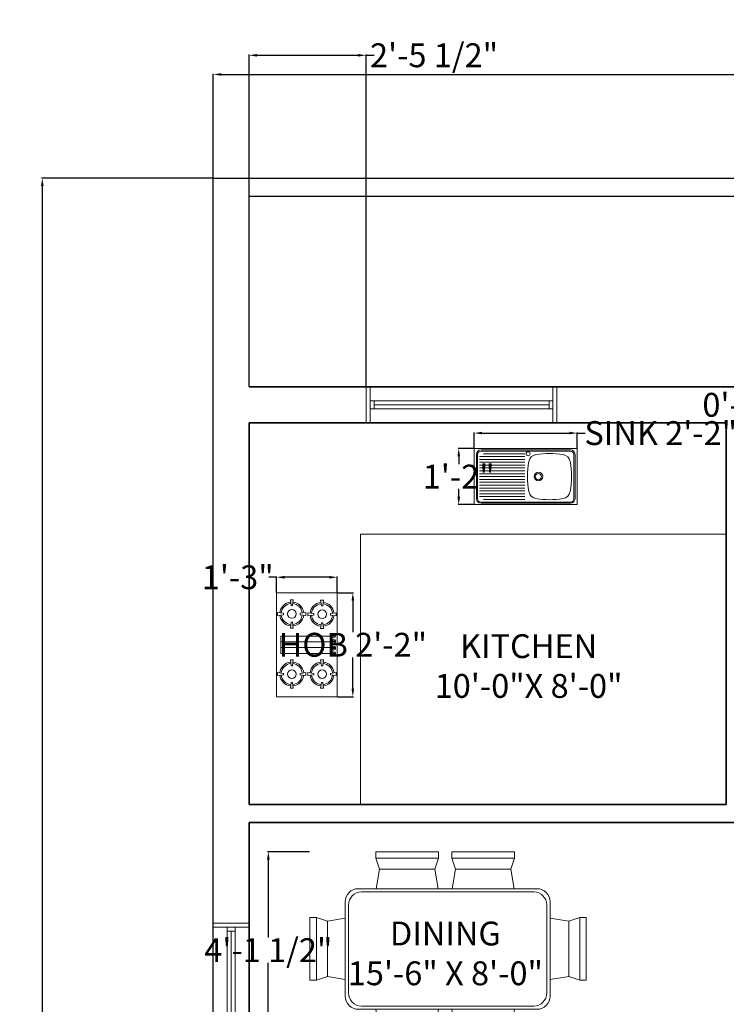
# Model space of a CAD drawing. Units: inches. Extents: x 84 to 590, y 32 to 648.
# Tile 5 of 6: x 84 to 262, y 401 to 648. Entities that reach past the tile are written whole.
import ezdxf

# ---------------------------------------------------------------- set-up
doc = ezdxf.new("R2010")
doc.units = ezdxf.units.IN
doc.header["$MEASUREMENT"] = 0
for name, color, linetype, lineweight in [('A-ANNO-DIMS', 2, 'Continuous', 18), ('A-AREA-IDEN', 7, 'Continuous', 18), ('A-EQPM', 9, 'Continuous', 18), ('A-FLOR-CASE', 9, 'Continuous', 18), ('A-FLOR-FIXT', 9, 'Continuous', 18), ('A-FURN', 8, 'Continuous', 18), ('A-GLAZ', 4, 'Continuous', 18), ('A-WALL', 7, 'Continuous', 35), ('C-PROP', 7, 'Continuous', 30)]:
    doc.layers.add(name, color=color, linetype=linetype, lineweight=lineweight)
doc.styles.get("Standard").update_dxf_attribs({"font": 'arial.ttf'})
doc.dimstyles.get("Standard").update_dxf_attribs({"dimtxt": 6, "dimasz": 2, "dimexe": 0.18, "dimexo": 0.0625, "dimgap": 0.09, "dimtad": 0, "dimtih": 1, "dimtoh": 1, "dimdec": 0, "dimzin": 0, "dimdsep": 46, "dimlunit": 4, "dimtxsty": 'Standard', "dimcen": 0.09, "dimadec": 0, "dimazin": 0, "dimtfac": 1, "dimtdec": 0, "dimtofl": 0, "dimtmove": 0, "dimatfit": 3, "dimfxl": 1, "dimtolj": 1, "dimtzin": 0, "dimarcsym": 1})

# ---------------------------------------------------------------- blocks, each defined once
blk = doc.blocks.new('A$C6C037A94')
for p, q in [((0.7877, 1.6959), (0.4032, 1.6959)), ((0.4032, 1.6959), (0.4039, 1.6557)), ((0.7877, 1.6557), (0.7877, 1.6959)), ((0.4258, 1.588), (0.4039, 1.6557)), ((0.7877, 1.6557), (0.4039, 1.6557)), ((0.7658, 1.588), (0.7877, 1.6557)), ((0.407, 1.4737), (0.4258, 1.588)), ((0.7658, 1.588), (0.4258, 1.588)), ((0.7847, 1.4737), (0.7658, 1.588)), ((0.307, 1.4737), (0.8868, 1.4737)), ((0.327, 1.4537), (0.8668, 1.4537)), ((0.227, 0.2974), (0.227, 1.3937)), ((0.9668, 1.3937), (0.9668, 0.2974)), ((0.247, 0.3174), (0.247, 1.3737)), ((0.9468, 1.3737), (0.9468, 0.3174)), ((0, 1.2552), (0, 0.8707)), ((0.0402, 1.2552), (0, 1.2552)), ((0.0402, 1.2552), (0.0402, 0.8714)), ((0.1079, 1.2333), (0.0402, 1.2552)), ((0.227, 1.2529), (0.1079, 1.2333)), ((0.1079, 1.2333), (0.1079, 0.8933)), ((0.9668, 1.2553), (1.1005, 1.2333)), ((1.1005, 1.2333), (1.1682, 1.2552)), ((1.1005, 1.2333), (1.1005, 0.8933)), ((1.1682, 1.2552), (1.2084, 1.2552)), ((1.1682, 1.2552), (1.1682, 0.8714)), ((1.2084, 1.2552), (1.2084, 0.8707)), ((0, 0.8707), (0.0402, 0.8714)), ((0.1079, 0.8933), (0.0402, 0.8714)), ((0.227, 0.8736), (0.1079, 0.8933)), ((0.9668, 0.8712), (1.1005, 0.8933)), ((1.1005, 0.8933), (1.1682, 0.8714)), ((1.2084, 0.8707), (1.1682, 0.8714)), ((0, 0.7888), (0, 0.4043)), ((0.0402, 0.7888), (0, 0.7888)), ((0.0402, 0.7888), (0.0402, 0.405)), ((0.1079, 0.7669), (0.0402, 0.7888)), ((0.227, 0.7865), (0.1079, 0.7669)), ((0.9668, 0.7889), (1.1005, 0.7669)), ((1.1005, 0.7669), (1.1682, 0.7888)), ((1.1682, 0.7888), (1.1682, 0.405)), ((1.1682, 0.7888), (1.2084, 0.7888)), ((1.2084, 0.7888), (1.2084, 0.4043)), ((0.1079, 0.7669), (0.1079, 0.4269)), ((1.1005, 0.7669), (1.1005, 0.4269)), ((0.1079, 0.4269), (0.0402, 0.405)), ((0.227, 0.4072), (0.1079, 0.4269)), ((0.9668, 0.4048), (1.1005, 0.4269)), ((1.1005, 0.4269), (1.1682, 0.405)), ((0, 0.4043), (0.0402, 0.405)), ((1.2084, 0.4043), (1.1682, 0.405)), ((0.8868, 0.2174), (0.307, 0.2174)), ((0.8668, 0.2374), (0.327, 0.2374)), ((0.4078, 0.2174), (0.4258, 0.1079)), ((0.7839, 0.2174), (0.7658, 0.1079)), ((0.4258, 0.1079), (0.4039, 0.0402)), ((0.7658, 0.1079), (0.4258, 0.1079)), ((0.7658, 0.1079), (0.7877, 0.0402)), ((0.4032, 0), (0.4039, 0.0402)), ((0.7877, 0), (0.4032, 0)), ((0.7877, 0.0402), (0.4039, 0.0402)), ((0.7877, 0.0402), (0.7877, 0))]:
    blk.add_line(p, q)
for centre, start, end in [((0.307, 1.3937), 90, 180), ((0.327, 1.3737), 90, 180), ((0.8668, 1.3737), 360, 90), ((0.8868, 1.3937), 360, 90), ((0.327, 0.3174), 180, 270), ((0.8668, 0.3174), 270, 0), ((0.307, 0.2974), 180, 270), ((0.8868, 0.2974), 270, 360)]:
    blk.add_arc(centre, 0.08, start, end)
blk = doc.blocks.new('A$C57CF26DA')
for p, q in [((0, 0), (0, 420)), ((720, 420), (0, 420)), ((166.9, 413), (146.9, 413)), ((146.9, 413), (151.9, 373)), ((161.9, 373), (166.9, 413)), ((583.6, 413), (563.6, 413)), ((563.6, 413), (568.6, 373)), ((578.6, 373), (583.6, 413)), ((720, 0), (720, 420)), ((151.9, 373), (161.9, 373)), ((300, 390.9), (300, 49.1)), ((300, 390.9), (420, 390.9)), ((340, 390.9), (340, 49.1)), ((380, 390.9), (380, 49.1)), ((420, 390.9), (420, 49.1)), ((568.6, 373), (578.6, 373)), ((98.9, 320), (58.9, 325)), ((58.9, 325), (58.9, 305)), ((58.9, 305), (98.9, 310)), ((98.9, 310), (98.9, 320)), ((254.8, 325), (214.8, 320)), ((214.8, 320), (214.8, 310)), ((214.8, 310), (254.8, 305)), ((254.8, 305), (254.8, 325)), ((515.6, 320), (475.6, 325)), ((475.6, 325), (475.6, 305)), ((475.6, 305), (515.6, 310)), ((515.6, 310), (515.6, 320)), ((671.6, 325), (631.6, 320)), ((631.6, 320), (631.6, 310)), ((631.6, 310), (671.6, 305)), ((671.6, 305), (671.6, 325)), ((151.9, 257), (146.9, 217)), ((146.9, 217), (166.9, 217)), ((161.9, 257), (151.9, 257)), ((166.9, 217), (161.9, 257)), ((568.6, 257), (563.6, 217)), ((563.6, 217), (583.6, 217)), ((578.6, 257), (568.6, 257)), ((583.6, 217), (578.6, 257)), ((166.9, 203), (146.9, 203)), ((146.9, 203), (151.9, 163)), ((151.9, 163), (161.9, 163)), ((161.9, 163), (166.9, 203)), ((581.1, 203), (561.1, 203)), ((561.1, 203), (566.1, 163)), ((566.1, 163), (576.1, 163)), ((576.1, 163), (581.1, 203)), ((98.9, 110), (58.9, 115)), ((58.9, 115), (58.9, 95)), ((58.9, 95), (98.9, 100)), ((98.9, 100), (98.9, 110)), ((254.8, 115), (214.8, 110)), ((214.8, 110), (214.8, 100)), ((214.8, 100), (254.8, 95)), ((254.8, 95), (254.8, 115)), ((513.1, 110), (473.1, 115)), ((473.1, 115), (473.1, 95)), ((473.1, 95), (513.1, 100)), ((513.1, 100), (513.1, 110)), ((669, 115), (629, 110)), ((629, 110), (629, 100)), ((629, 100), (669, 95)), ((669, 95), (669, 115)), ((151.9, 47), (146.9, 7)), ((146.9, 7), (166.9, 7)), ((161.9, 47), (151.9, 47)), ((166.9, 7), (161.9, 47)), ((301.5, 38.7), (294.7, 38.7)), ((294.7, 38.7), (294.7, 11.3)), ((294.7, 11.3), (301.5, 11.3)), ((420, 49.1), (300, 49.1)), ((301.5, 11.3), (301.5, 38.7)), ((340.5, 38.7), (333.7, 38.7)), ((333.7, 38.7), (333.7, 11.3)), ((333.7, 11.3), (340.5, 11.3)), ((340.5, 11.3), (340.5, 38.7)), ((379.7, 11.3), (379.7, 38.7)), ((379.7, 38.7), (386.5, 38.7)), ((386.5, 11.3), (379.7, 11.3)), ((386.5, 38.7), (386.5, 11.3)), ((418.7, 11.3), (418.7, 38.7)), ((418.7, 38.7), (425.5, 38.7)), ((425.5, 11.3), (418.7, 11.3)), ((425.5, 38.7), (425.5, 11.3)), ((566.1, 47), (561.1, 7)), ((561.1, 7), (581.1, 7)), ((576.1, 47), (566.1, 47)), ((581.1, 7), (576.1, 47)), ((720, 0), (0, 0))]:
    blk.add_line(p, q)
for centre in [(156.9, 315), (573.6, 315), (156.9, 105), (571.1, 105)]:
    blk.add_circle(centre, 30)
for centre, radius, start, end in [((156.9, 315), 83, 95.58493, 174.41507), ((156.9, 315), 73, 95.37384, 174.62616), ((156.9, 315), 73, 5.37384, 84.62616), ((156.9, 315), 83, 5.58493, 84.41507), ((573.6, 315), 83, 95.58493, 174.41507), ((573.6, 315), 73, 95.37384, 174.62616), ((573.6, 315), 73, 5.37384, 84.62616), ((573.6, 315), 83, 5.58493, 84.41507), ((156.9, 315), 83, 185.58493, 264.41507), ((156.9, 315), 73, 185.37384, 264.62616), ((156.9, 315), 73, 275.37384, 354.62616), ((156.9, 315), 83, 275.58493, 354.41507), ((573.6, 315), 83, 185.58493, 264.41507), ((573.6, 315), 73, 185.37384, 264.62616), ((573.6, 315), 73, 275.37384, 354.62616), ((573.6, 315), 83, 275.58493, 354.41507), ((156.9, 105), 83, 95.58493, 174.41507), ((156.9, 105), 73, 95.37384, 174.62616), ((156.9, 105), 73, 5.37384, 84.62616), ((156.9, 105), 83, 5.58493, 84.41507), ((571.1, 105), 83, 95.58493, 174.41507), ((571.1, 105), 73, 95.37384, 174.62616), ((571.1, 105), 73, 5.37384, 84.62616), ((571.1, 105), 83, 5.58493, 84.41507), ((156.9, 105), 83, 185.58493, 264.41507), ((156.9, 105), 73, 185.37384, 264.62616), ((156.9, 105), 73, 275.37384, 354.62616), ((156.9, 105), 83, 275.58493, 354.41507), ((571.1, 105), 83, 185.58493, 264.41507), ((571.1, 105), 73, 185.37384, 264.62616), ((571.1, 105), 73, 275.37384, 354.62616), ((571.1, 105), 83, 275.58493, 354.41507), ((298.1, 25), 13.7, 104.47751, 255.52249), ((298.1, 25), 13.7, 284.47751, 75.52249), ((337.1, 25), 13.7, 104.47751, 255.52249), ((337.1, 25), 13.7, 284.47751, 75.52249), ((383.1, 25), 13.7, 104.47751, 255.52249), ((383.1, 25), 13.7, 284.47751, 75.52249), ((422.1, 25), 13.7, 104.47751, 255.52249), ((422.1, 25), 13.7, 284.47751, 75.52249)]:
    blk.add_arc(centre, radius, start, end)
blk = doc.blocks.new('A$C0C3933DC')
for p, q in [((0, 490), (0, 0)), ((900, 490), (0, 490)), ((19.5, 52.5), (19.5, 437.5)), ((29.5, 52.5), (29.5, 437.5)), ((59.5, 477.5), (450, 477.5)), ((59.5, 467.5), (450, 467.5)), ((441, 445), (80.7, 445)), ((840.5, 477.5), (450, 477.5)), ((840.5, 467.5), (450, 467.5)), ((870.5, 52.5), (870.5, 437.5)), ((880.5, 52.5), (880.5, 437.5)), ((900, 0), (900, 490)), ((441, 420), (45, 420)), ((441, 395), (45, 395)), ((441, 370), (45, 370)), ((441, 345), (45, 345)), ((441, 320), (45, 320)), ((441, 295), (45, 295)), ((441, 270), (45, 270)), ((441, 245), (45, 245)), ((441, 220), (45, 220)), ((441, 195), (45, 195)), ((441, 170), (45, 170)), ((441, 145), (45, 145)), ((441, 120), (45, 120)), ((441, 95), (45, 95)), ((0, 0), (900, 0)), ((441, 70), (45, 70)), ((450, 22.5), (59.5, 22.5)), ((450, 12.5), (59.5, 12.5)), ((441, 45), (80.7, 45)), ((450, 22.5), (840.5, 22.5)), ((450, 12.5), (840.5, 12.5))]:
    blk.add_line(p, q)
for centre, radius in [((471, 445), 17.5), ((561, 245), 38), ((561, 245), 27.5)]:
    blk.add_circle(centre, radius)
for centre, radius, start, end in [((59.5, 437.5), 40, 90, 180), ((59.5, 437.5), 30, 90, 180), ((551.5, 363.5), 75, 99.07872, 169.88522), ((658, -303), 750, 80.92128, 99.07872), ((764.5, 363.5), 75, 10.11478, 80.92128), ((840.5, 437.5), 40, 0, 90), ((840.5, 437.5), 30, 0, 90), ((1216, 245), 750, 169.88522, 190.11478), ((100, 245), 750, 349.88522, 10.11478), ((551.5, 126.5), 75, 190.11478, 260.92128), ((764.5, 126.5), 75, 279.07872, 349.88522), ((59.5, 52.5), 40, 180, 270), ((59.5, 52.5), 30, 180, 270), ((658, 793), 750, 260.92128, 279.07872), ((840.5, 52.5), 30, 270, 0), ((840.5, 52.5), 40, 270, 0)]:
    blk.add_arc(centre, radius, start, end)
blk = doc.blocks.new('*D12')
at = {"layer": 'A-ANNO-DIMS', "color": 0, "lineweight": -2, "transparency": 16777216}
for p, q in [((133.03, 608.4), (133.03, 634.6)), ((135.03, 634.42), (307.85, 634.42)), ((491.03, 634.42), (318.21, 634.42)), ((493.03, 608.4), (493.03, 634.6))]:
    blk.add_line(p, q, dxfattribs=at)
at = {"layer": 'A-ANNO-DIMS', "color": 0, "transparency": 16777216}
for points in [[(135.03, 634.75), (135.03, 634.08), (133.03, 634.42)], [(491.03, 634.75), (491.03, 634.08), (493.03, 634.42)]]:
    blk.add_solid(points, dxfattribs=at)
at = {"layer": 'Defpoints', "color": 0, "transparency": 16777216}
for p in [(493.03, 634.42), (133.03, 608.34), (493.03, 608.34)]:
    blk.add_point(p, dxfattribs=at)
at = {"layer": 'A-ANNO-DIMS', "color": 0, "transparency": 16777216, "insert": (313.03, 634.42), "char_height": 6, "attachment_point": 5}
blk.add_mtext("\\A1;30'", dxfattribs=at)
blk = doc.blocks.new('*D13')
at = {"layer": 'A-ANNO-DIMS', "color": 0, "lineweight": -2, "transparency": 16777216}
for p, q in [((132.97, 608.34), (89.87, 608.34)), ((90.05, 606.34), (90.05, 359.49)), ((90.05, 106.34), (90.05, 353.18)), ((132.97, 104.34), (89.87, 104.34))]:
    blk.add_line(p, q, dxfattribs=at)
at = {"layer": 'A-ANNO-DIMS', "color": 0, "transparency": 16777216}
for points in [[(89.71, 606.34), (90.38, 606.34), (90.05, 608.34)], [(89.71, 106.34), (90.38, 106.34), (90.05, 104.34)]]:
    blk.add_solid(points, dxfattribs=at)
at = {"layer": 'Defpoints', "color": 0, "transparency": 16777216}
for p in [(90.05, 608.34), (133.03, 608.34), (133.03, 104.34)]:
    blk.add_point(p, dxfattribs=at)
at = {"layer": 'A-ANNO-DIMS', "color": 0, "transparency": 16777216, "insert": (90.05, 356.34), "char_height": 6, "attachment_point": 5}
blk.add_mtext("\\A1;40'", dxfattribs=at)
blk = doc.blocks.new('WIND')
for p, q in [((-51.89, 1021.98), (-99.89, 1021.98)), ((-99.89, 1021.98), (-99.89, 1012.98)), ((-98.89, 1021.98), (-98.89, 1012.98)), ((-52.89, 1012.98), (-52.89, 1021.98)), ((-51.89, 1012.98), (-51.89, 1021.98)), ((-98.89, 1018.48), (-52.89, 1018.48)), ((-97.89, 1018.48), (-97.89, 1016.48)), ((-53.89, 1016.48), (-53.89, 1018.48)), ((-98.89, 1016.48), (-52.89, 1016.48)), ((-97.89, 1017.48), (-53.89, 1017.48)), ((-99.89, 1012.98), (-51.89, 1012.98))]:
    blk.add_line(p, q)
blk = doc.blocks.new('*D20')
at = {"layer": 'A-ANNO-DIMS', "color": 0, "lineweight": -2, "transparency": 16777216}
for p, q in [((274.33, 557.84), (274.33, 559.84)), ((277.86, 555.84), (274.15, 555.84)), ((277.86, 546.84), (274.15, 546.84)), ((274.33, 544.84), (274.33, 542.84))]:
    blk.add_line(p, q, dxfattribs=at)
at = {"layer": 'A-ANNO-DIMS', "color": 0, "transparency": 16777216}
for points in [[(273.99, 557.84), (274.66, 557.84), (274.33, 555.84)], [(273.99, 544.84), (274.66, 544.84), (274.33, 546.84)]]:
    blk.add_solid(points, dxfattribs=at)
at = {"layer": 'Defpoints', "color": 0, "transparency": 16777216}
for p in [(274.33, 555.84), (277.93, 555.84), (277.93, 546.84)]:
    blk.add_point(p, dxfattribs=at)
at = {"layer": 'A-ANNO-DIMS', "color": 0, "transparency": 16777216, "insert": (274.33, 551.34), "char_height": 6, "attachment_point": 5}
blk.add_mtext('\\A1;0\'-9" TYP.', dxfattribs=at)
blk = doc.blocks.new('*D32')
at = {"layer": 'A-ANNO-DIMS', "color": 0, "lineweight": -2, "transparency": 16777216}
for p, q in [((157.25, 438.96), (146.7, 438.96)), ((146.88, 436.96), (146.88, 417.39)), ((146.88, 391.43), (146.88, 411)), ((157.25, 389.43), (146.7, 389.43))]:
    blk.add_line(p, q, dxfattribs=at)
at = {"layer": 'A-ANNO-DIMS', "color": 0, "transparency": 16777216}
for points in [[(146.55, 436.96), (147.22, 436.96), (146.88, 438.96)], [(146.55, 391.43), (147.22, 391.43), (146.88, 389.43)]]:
    blk.add_solid(points, dxfattribs=at)
at = {"layer": 'Defpoints', "color": 0, "transparency": 16777216}
for p in [(157.31, 438.96), (146.88, 389.43), (157.31, 389.43)]:
    blk.add_point(p, dxfattribs=at)
at = {"layer": 'A-ANNO-DIMS', "color": 0, "transparency": 16777216, "insert": (146.88, 414.2), "char_height": 6, "attachment_point": 5}
blk.add_mtext('\\A1;4\'-1 1/2"', dxfattribs=at)
blk = doc.blocks.new('*D33')
at = {"layer": 'A-ANNO-DIMS', "color": 0, "lineweight": -2, "transparency": 16777216}
for p, q in [((164.27, 504.06), (168.31, 504.06)), ((168.13, 502.06), (168.13, 494.19)), ((168.13, 479.94), (168.13, 487.81)), ((164.27, 477.94), (168.31, 477.94))]:
    blk.add_line(p, q, dxfattribs=at)
at = {"layer": 'A-ANNO-DIMS', "color": 0, "transparency": 16777216}
for points in [[(167.79, 502.06), (168.46, 502.06), (168.13, 504.06)], [(167.79, 479.94), (168.46, 479.94), (168.13, 477.94)]]:
    blk.add_solid(points, dxfattribs=at)
at = {"layer": 'Defpoints', "color": 0, "transparency": 16777216}
for p in [(164.21, 504.06), (168.13, 504.06), (164.21, 477.94)]:
    blk.add_point(p, dxfattribs=at)
at = {"layer": 'A-ANNO-DIMS', "color": 0, "transparency": 16777216, "insert": (168.13, 491), "char_height": 6, "attachment_point": 5}
blk.add_mtext('\\A1;HOB 2\'-2"', dxfattribs=at)
blk = doc.blocks.new('*D34')
at = {"layer": 'A-ANNO-DIMS', "color": 0, "lineweight": -2, "transparency": 16777216}
for p, q in [((148.97, 507.98), (146.97, 507.98)), ((148.97, 504.12), (148.97, 508.16)), ((162.21, 507.98), (150.97, 507.98)), ((164.21, 504.12), (164.21, 508.16))]:
    blk.add_line(p, q, dxfattribs=at)
at = {"layer": 'A-ANNO-DIMS', "color": 0, "transparency": 16777216}
for points in [[(150.97, 508.31), (150.97, 507.64), (148.97, 507.98)], [(162.21, 508.31), (162.21, 507.64), (164.21, 507.98)]]:
    blk.add_solid(points, dxfattribs=at)
at = {"layer": 'Defpoints', "color": 0, "transparency": 16777216}
for p in [(148.97, 507.98), (148.97, 504.06), (164.21, 504.06)]:
    blk.add_point(p, dxfattribs=at)
at = {"layer": 'A-ANNO-DIMS', "color": 0, "transparency": 16777216, "insert": (139.19, 507.98), "char_height": 6, "attachment_point": 5}
blk.add_mtext('\\A1;1\'-3"', dxfattribs=at)
blk = doc.blocks.new('*D35')
at = {"layer": 'A-ANNO-DIMS', "color": 0, "lineweight": -2, "transparency": 16777216}
for p, q in [((198.64, 540.41), (198.64, 544.41)), ((200.64, 544.23), (222.55, 544.23)), ((224.55, 540.41), (224.55, 544.41)), ((224.55, 544.23), (226.55, 544.23))]:
    blk.add_line(p, q, dxfattribs=at)
at = {"layer": 'A-ANNO-DIMS', "color": 0, "transparency": 16777216}
for points in [[(200.64, 544.57), (200.64, 543.9), (198.64, 544.23)], [(222.55, 544.57), (222.55, 543.9), (224.55, 544.23)]]:
    blk.add_solid(points, dxfattribs=at)
at = {"layer": 'Defpoints', "color": 0, "transparency": 16777216}
for p in [(224.55, 544.23), (198.64, 540.35), (224.55, 540.35)]:
    blk.add_point(p, dxfattribs=at)
at = {"layer": 'A-ANNO-DIMS', "color": 0, "transparency": 16777216, "insert": (245.55, 544.23), "char_height": 6, "attachment_point": 5}
blk.add_mtext('\\A1;SINK 2\'-2"', dxfattribs=at)
blk = doc.blocks.new('*D36')
at = {"layer": 'A-ANNO-DIMS', "color": 0, "lineweight": -2, "transparency": 16777216}
for p, q in [((198.58, 540.35), (194.57, 540.35)), ((194.75, 538.35), (194.75, 536.4)), ((194.75, 528.24), (194.75, 530.19)), ((198.58, 526.24), (194.57, 526.24))]:
    blk.add_line(p, q, dxfattribs=at)
at = {"layer": 'A-ANNO-DIMS', "color": 0, "transparency": 16777216}
for points in [[(194.42, 538.35), (195.09, 538.35), (194.75, 540.35)], [(194.42, 528.24), (195.09, 528.24), (194.75, 526.24)]]:
    blk.add_solid(points, dxfattribs=at)
at = {"layer": 'Defpoints', "color": 0, "transparency": 16777216}
for p in [(194.75, 540.35), (198.64, 540.35), (198.64, 526.24)]:
    blk.add_point(p, dxfattribs=at)
at = {"layer": 'A-ANNO-DIMS', "color": 0, "transparency": 16777216, "insert": (194.75, 533.29), "char_height": 6, "attachment_point": 5}
blk.add_mtext('\\A1;1\'-2"', dxfattribs=at)
blk = doc.blocks.new('*D49')
at = {"layer": 'A-ANNO-DIMS', "color": 0, "lineweight": -2, "transparency": 16777216}
for p, q in [((142.03, 555.9), (142.03, 639.42)), ((144.03, 639.24), (169.45, 639.24)), ((171.45, 555.9), (171.45, 639.42)), ((171.45, 639.24), (173.45, 639.24))]:
    blk.add_line(p, q, dxfattribs=at)
at = {"layer": 'A-ANNO-DIMS', "color": 0, "transparency": 16777216}
for points in [[(144.03, 639.57), (144.03, 638.9), (142.03, 639.24)], [(169.45, 639.57), (169.45, 638.9), (171.45, 639.24)]]:
    blk.add_solid(points, dxfattribs=at)
at = {"layer": 'Defpoints', "color": 0, "transparency": 16777216}
for p in [(171.45, 639.24), (142.03, 555.84), (171.45, 555.84)]:
    blk.add_point(p, dxfattribs=at)
at = {"layer": 'A-ANNO-DIMS', "color": 0, "transparency": 16777216, "insert": (188.55, 639.24), "char_height": 6, "attachment_point": 5}
blk.add_mtext('\\A1;2\'-5 1/2"', dxfattribs=at)

msp = doc.modelspace()

# ---------------------------------------------------------------- linework, layer by layer
at = {"layer": 'A-FLOR-CASE'}
for p, q in [((170.03, 518.84), (262.03, 518.84)), ((170.03, 450.84), (170.03, 518.84))]:
    msp.add_line(p, q, dxfattribs=at)
at = {"layer": 'A-WALL'}
for p, q in [((142.03, 555.84), (484.03, 555.84)), ((142.03, 546.84), (262.03, 546.84)), ((142.03, 450.84), (142.03, 546.84)), ((262.03, 450.84), (262.03, 546.84)), ((142.03, 450.84), (262.03, 450.84)), ((142.03, 446.34), (269.53, 446.34)), ((142.03, 254.34), (142.03, 446.34))]:
    msp.add_line(p, q, dxfattribs=at)
at = {"layer": 'C-PROP'}
for p, q in [((133.03, 608.34), (493.03, 608.34)), ((133.03, 104.34), (133.03, 608.34)), ((142.03, 603.84), (484.03, 603.84)), ((142.03, 555.84), (142.03, 603.84))]:
    msp.add_line(p, q, dxfattribs=at)

# ---------------------------------------------------------------- block references
at = {"layer": 'A-EQPM', "xscale": 0.0362780453766686, "yscale": 0.0362780453766686, "zscale": 0.0362780453766686, "rotation": 90}
msp.add_blockref('A$C57CF26DA', (164.21, 477.94), dxfattribs=at)
at = {"layer": 'A-FLOR-FIXT', "xscale": 0.0287900870179948, "yscale": 0.0287900870179948, "zscale": 0.0287900870179948}
msp.add_blockref('A$C0C3933DC', (198.64, 526.24), dxfattribs=at)
at = {"layer": 'A-FURN', "xscale": 40.98563321974356, "yscale": 40.98563321974356, "zscale": 40.98563321974356, "rotation": 270}
msp.add_blockref('A$C6C037A94', (157.31, 438.96), dxfattribs=at)
at = {"layer": 'A-GLAZ'}
msp.add_blockref('WIND', (271.34, -466.14), dxfattribs=at)
at = {"layer": 'A-GLAZ', "rotation": 270}
msp.add_blockref('WIND', (-879.95, 321.13), dxfattribs=at)

# ---------------------------------------------------------------- texts
at = {"layer": 'A-AREA-IDEN', "char_height": 6, "attachment_point": 1}
for s, width, insert in [('\\pxqc;KITCHEN\\P10\'-0"X 8\'-0"', 93.8598, (165.39, 493.65)), ('\\pxqc;DINING\\P15\'-6" X 8\'-0"', 115.0687, (133.86, 421.39))]:
    msp.add_mtext_dynamic_manual_height_columns(s, width=width, gutter_width=30, heights=[0], dxfattribs=dict(at, insert=insert))

# ---------------------------------------------------------------- dimensions: what is measured, and where the dimension line sits
at = {"layer": 'A-ANNO-DIMS'}
for base, p1, p2, override, picture, middle in [((171.45, 639.24), (142.03, 555.84), (171.45, 555.84), {"dimdec": 1, "dimlfac": 1, "dimrnd": 0, "dimzin": 1, "dimdsep": 46, "dimlunit": 4, "dimfrac": 2}, '*D49', (188.55, 639.24)), ((493.03, 634.42), (133.03, 608.34), (493.03, 608.34), {"dimclrd": 0, "dimclre": 0, "dimclrt": 0}, '*D12', (313.03, 634.42))]:
    dim = msp.add_linear_dim(base=base, p1=p1, p2=p2, dimstyle='Standard', override=override, dxfattribs=at)
    dim.commit()
    dim.dimension.update_dxf_attribs({"geometry": picture, "text_midpoint": middle})
for base, p1, p2, text, override, picture, middle in [((90.05, 608.34), (133.03, 104.34), (133.03, 608.34), "40'", {"dimclrd": 0, "dimclre": 0, "dimclrt": 0}, '*D13', (90.05, 356.34)), ((274.33, 555.84), (277.93, 546.84), (277.93, 555.84), '<> TYP.', {"dimdec": 1, "dimlfac": 1, "dimrnd": 0, "dimzin": 1, "dimdsep": 46, "dimlunit": 4, "dimfrac": 2}, '*D20', (274.33, 551.34)), ((168.13, 504.06), (164.21, 477.94), (164.21, 504.06), 'HOB <>', {"dimdec": 1, "dimlfac": 1, "dimrnd": 0, "dimzin": 1, "dimdsep": 46, "dimlunit": 4, "dimfrac": 2}, '*D33', (168.13, 491))]:
    dim = msp.add_linear_dim(base=base, p1=p1, p2=p2, angle=90, text=text, dimstyle='Standard', override=override, dxfattribs=at)
    dim.commit()
    dim.dimension.update_dxf_attribs({"geometry": picture, "text_midpoint": middle})
dim = msp.add_linear_dim(base=(224.55, 544.23), p1=(198.64, 540.35), p2=(224.55, 540.35), text='SINK <>', dimstyle='Standard', override={"dimdec": 1, "dimlfac": 1, "dimrnd": 0, "dimzin": 1, "dimdsep": 46, "dimlunit": 4, "dimfrac": 2}, dxfattribs=at)
dim.commit()
dim.dimension.update_dxf_attribs({"geometry": '*D35', "text_midpoint": (245.55, 544.23)})
for base, p1, p2, angle, picture, middle in [((194.75, 540.35), (198.64, 526.24), (198.64, 540.35), 90, '*D36', (194.75, 533.29)), ((148.97, 507.98), (164.21, 504.06), (148.97, 504.06), 180, '*D34', (139.19, 507.98)), ((146.88, 389.43), (157.31, 438.96), (157.31, 389.43), 270, '*D32', (146.88, 414.2))]:
    dim = msp.add_linear_dim(base=base, p1=p1, p2=p2, angle=angle, dimstyle='Standard', override={"dimdec": 1, "dimlfac": 1, "dimrnd": 0, "dimzin": 1, "dimdsep": 46, "dimlunit": 4, "dimfrac": 2}, dxfattribs=at)
    dim.commit()
    dim.dimension.update_dxf_attribs({"geometry": picture, "text_midpoint": middle})

doc.saveas('drawing.dxf')
